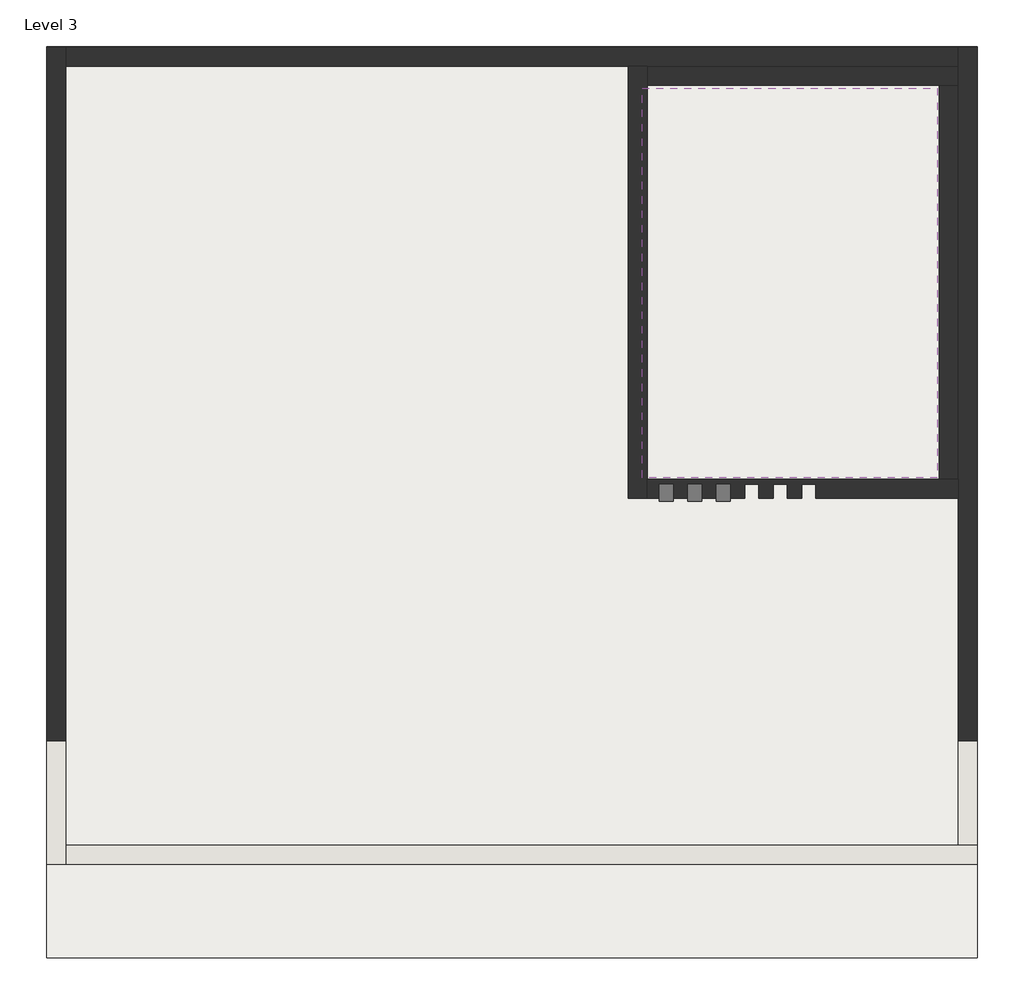
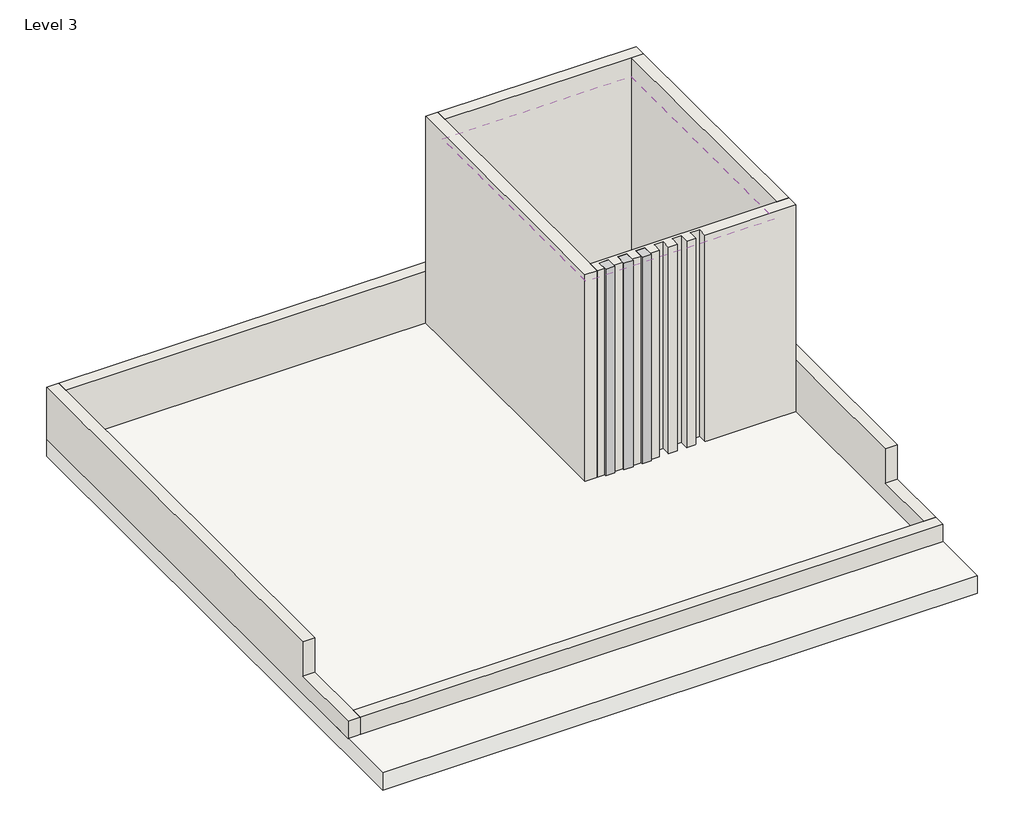
# One storey, incomplete: 8 walls, 3 proxies, 2 roofs.
"""IFC4 building model written with IfcOpenShell, lengths in millimetres."""

from ifc_helpers import new_model, si_unit, frame, origin, place, context, project, spatial, polyline, outline, extrude, faceted_brep, element, save

model = new_model("IFC4")

# Units and contexts
model_context = context("Model", 3, world=origin())
ifc_project = project(units=[si_unit("LENGTHUNIT", "METRE", prefix="MILLI")], contexts=[model_context])

# Site, building, storey
site = spatial("IfcSite", under=ifc_project)
building = spatial("IfcBuilding", under=site)
storey = spatial("IfcBuildingStorey", under=building, Name="Level 3", Elevation=7315.2)

# Proxies
placement = place(None, origin())
element("IfcBuildingElementProxy", 1, Name="Reveal", ObjectType="Reveal", at=placement, inside=storey, context=model_context, shape_type="SweptSolid", body=[
    extrude(outline(polyline([(-6259.9931367, 6437.3997066), (-6259.9931367, 6620.2797066), (-6107.5931367, 6620.2797066), (-6107.5931367, 6437.3997066), (-6259.9931367, 6437.3997066)])), frame((0.0, 0.0, 7620.0), z_axis=(0.0, 0.0, 1.0), x_axis=(1.0, 0.0, 0.0)), (0.0, 0.0, 1.0), 3657.6),
])
element("IfcBuildingElementProxy", 2, Name="Reveal", ObjectType="Reveal", at=placement, inside=storey, context=model_context, shape_type="SweptSolid", body=[
    extrude(outline(polyline([(-5955.1931367, 6437.3997066), (-5955.1931367, 6620.2797066), (-5802.7931367, 6620.2797066), (-5802.7931367, 6437.3997066), (-5955.1931367, 6437.3997066)])), frame((0.0, 0.0, 7620.0), z_axis=(0.0, 0.0, 1.0), x_axis=(1.0, 0.0, 0.0)), (0.0, 0.0, 1.0), 3657.6),
])
element("IfcBuildingElementProxy", 3, Name="Reveal", ObjectType="Reveal", at=placement, inside=storey, context=model_context, shape_type="SweptSolid", body=[
    extrude(outline(polyline([(-5650.3931367, 6437.3997066), (-5650.3931367, 6620.2797066), (-5497.9931367, 6620.2797066), (-5497.9931367, 6437.3997066), (-5650.3931367, 6437.3997066)])), frame((0.0, 0.0, 7620.0), z_axis=(0.0, 0.0, 1.0), x_axis=(1.0, 0.0, 0.0)), (0.0, 0.0, 1.0), 3657.6),
])

# Roofs
element("IfcRoof", 4, ObjectType="Generic - 12\"", at=placement, inside=storey, context=model_context, shape_type="SweptSolid", body=[
    extrude(outline(polyline([(-12813.1931367, 11300.8300502), (-2856.3931367, 11300.8300502), (-2856.3931367, 1552.6285778), (-12813.1931367, 1552.6285778), (-12813.1931367, 11300.8300502)])), frame((0.0, 0.0, 7315.2), z_axis=(0.0, 0.0, 1.0), x_axis=(1.0, 0.0, 0.0)), (0.0, 0.0, 1.0), 304.8),
])
element("IfcRoof", 5, ObjectType="Generic - 12\"", at=placement, inside=storey, context=model_context, shape_type="SweptSolid", body=[
    extrude(outline(polyline([(-6444.1431367, 10855.7297066), (-3288.1931367, 10855.7297066), (-3288.1931367, 6690.1297066), (-6444.1431367, 6690.1297066), (-6444.1431367, 10855.7297066)])), frame((0.0, 0.0, 10972.8), z_axis=(0.0, 0.0, 1.0), x_axis=(1.0, 0.0, 0.0)), (0.0, 0.0, 1.0), 304.8),
])

# Walls
element("IfcWall", 6, ObjectType="Generic - 8\"", at=placement, inside=storey, context=model_context, shape_type="Brep", body=[
    faceted_brep([(-12813.1931367, 11293.8797066, 7620.0), (-12813.1931367, 2556.2797066, 7620.0), (-12813.1931367, 2556.2797066, 7924.8), (-12813.1931367, 3877.0797066, 7924.8), (-12813.1931367, 3877.0797066, 8534.4), (-12813.1931367, 11293.8797066, 8534.4), (-12609.9931367, 11293.8797066, 7620.0), (-12609.9931367, 11293.8797066, 8534.4), (-12609.9931367, 11090.6797066, 8534.4), (-12609.9931367, 3877.0797066, 8534.4), (-12609.9931367, 3877.0797066, 7924.8), (-12609.9931367, 2759.4797066, 7924.8), (-12609.9931367, 2556.2797066, 7924.8), (-12609.9931367, 2556.2797066, 7620.0)], [[[0, 1, 2, 3, 4, 5]], [[6, 7, 8, 9, 10, 11, 12, 13]], [[2, 1, 13, 12]], [[0, 5, 7, 6]], [[1, 0, 6, 13]], [[5, 4, 9, 8, 7]], [[3, 2, 12, 11, 10]], [[4, 3, 10, 9]]]),
])
element("IfcWall", 7, ObjectType="Generic - 8\"", at=placement, inside=storey, context=model_context, shape_type="Brep", body=[
    faceted_brep([(-12609.9931367, 2556.2797066, 7315.2), (-2856.3931367, 2556.2797066, 7315.2), (-2856.3931367, 2556.2797066, 7924.8), (-12609.9931367, 2556.2797066, 7924.8), (-12609.9931367, 2556.2797066, 7620.0), (-12609.9931367, 2759.4797066, 7315.2), (-12609.9931367, 2759.4797066, 7924.8), (-3059.5931367, 2759.4797066, 7924.8), (-2856.3931367, 2759.4797066, 7924.8), (-2856.3931367, 2759.4797066, 7620.0), (-2856.3931367, 2759.4797066, 7315.2)], [[[0, 1, 2, 3, 4]], [[5, 6, 7, 8, 9, 10]], [[0, 4, 3, 6, 5]], [[2, 1, 10, 9, 8]], [[1, 0, 5, 10]], [[3, 2, 8, 7, 6]]]),
])
element("IfcWall", 8, ObjectType="Generic - 8\"", at=placement, inside=storey, context=model_context, shape_type="Brep", body=[
    faceted_brep([(-2856.3931367, 11293.8797066, 7620.0), (-2856.3931367, 11293.8797066, 8534.4), (-2856.3931367, 3877.0797066, 8534.4), (-2856.3931367, 3877.0797066, 7924.8), (-2856.3931367, 2759.4797066, 7924.8), (-2856.3931367, 2759.4797066, 7620.0), (-3059.5931367, 11293.8797066, 7620.0), (-3059.5931367, 2759.4797066, 7620.0), (-3059.5931367, 2759.4797066, 7924.8), (-3059.5931367, 3877.0797066, 7924.8), (-3059.5931367, 3877.0797066, 8534.4), (-3059.5931367, 11090.6797066, 8534.4), (-3059.5931367, 11293.8797066, 8534.4)], [[[0, 1, 2, 3, 4, 5]], [[6, 7, 8, 9, 10, 11, 12]], [[1, 0, 6, 12]], [[0, 5, 7, 6]], [[2, 1, 12, 11, 10]], [[3, 2, 10, 9]], [[4, 3, 9, 8]], [[5, 4, 8, 7]]]),
])
element("IfcWall", 9, ObjectType="Generic - 8\"", at=placement, inside=storey, context=model_context, shape_type="Brep", body=[
    faceted_brep([(-3059.5931367, 11293.8797066, 7315.2), (-12609.9931367, 11293.8797066, 7315.2), (-12609.9931367, 11293.8797066, 7620.0), (-12609.9931367, 11293.8797066, 8534.4), (-3059.5931367, 11293.8797066, 8534.4), (-3059.5931367, 11293.8797066, 7620.0), (-3059.5931367, 11090.6797066, 7315.2), (-3059.5931367, 11090.6797066, 8534.4), (-12609.9931367, 11090.6797066, 8534.4), (-12609.9931367, 11090.6797066, 7315.2)], [[[0, 1, 2, 3, 4, 5]], [[6, 7, 8, 9]], [[1, 0, 6, 9]], [[4, 3, 8, 7]], [[3, 2, 1, 9, 8]], [[0, 5, 4, 7, 6]]]),
])
element("IfcWall", 10, ObjectType="Generic - 8\"", at=placement, inside=storey, context=model_context, shape_type="Brep", body=[
    faceted_brep([(-6590.1931367, 11090.6797066, 11277.6), (-6590.1931367, 11090.6797066, 3962.4), (-6590.1931367, 6467.8797066, 3962.4), (-6590.1931367, 6467.8797066, 11277.6), (-6386.9931367, 11090.6797066, 3962.4), (-6386.9931367, 11090.6797066, 7315.2), (-6386.9931367, 11090.6797066, 11277.6), (-6386.9931367, 10887.4797066, 11277.6), (-6386.9931367, 6671.0797066, 11277.6), (-6386.9931367, 6467.8797066, 11277.6), (-6386.9931367, 6467.8797066, 3962.4), (-6386.9931367, 6671.0797066, 3962.4)], [[[0, 1, 2, 3]], [[4, 5, 6, 7, 8, 9, 10, 11]], [[2, 1, 4, 11, 10]], [[0, 3, 9, 8, 7, 6]], [[3, 2, 10, 9]], [[0, 6, 5, 4, 1]]]),
])
element("IfcWall", 11, ObjectType="Generic - 8\"", at=placement, inside=storey, context=model_context, shape_type="Brep", body=[
    faceted_brep([(-6386.9931367, 6467.8797066, 11277.6), (-6386.9931367, 6467.8797066, 3962.4), (-5345.5931367, 6467.8797066, 3962.4), (-5345.5931367, 6467.8797066, 11277.6), (-5497.9931367, 6467.8797066, 11277.6), (-5497.9931367, 6467.8797066, 7620.0), (-5650.3931367, 6467.8797066, 7620.0), (-5650.3931367, 6467.8797066, 11277.6), (-5802.7931367, 6467.8797066, 11277.6), (-5802.7931367, 6467.8797066, 7620.0), (-5955.1931367, 6467.8797066, 7620.0), (-5955.1931367, 6467.8797066, 11277.6), (-6107.5931367, 6467.8797066, 11277.6), (-6107.5931367, 6467.8797066, 7620.0), (-6259.9931367, 6467.8797066, 7620.0), (-6259.9931367, 6467.8797066, 11277.6), (-3059.5931367, 6467.8797066, 3962.4), (-3059.5931367, 6467.8797066, 11277.6), (-4583.5931367, 6467.8797066, 11277.6), (-4583.5931367, 6467.8797066, 3962.4), (-4431.1931367, 6467.8797066, 3962.4), (-4431.1931367, 6467.8797066, 7315.2), (-4278.7931367, 6467.8797066, 7315.2), (-4278.7931367, 6467.8797066, 3962.4), (-4126.3931367, 6467.8797066, 3962.4), (-4126.3931367, 6467.8797066, 7315.2), (-3973.9931367, 6467.8797066, 7315.2), (-3973.9931367, 6467.8797066, 3962.4), (-3821.5931367, 6467.8797066, 3962.4), (-3821.5931367, 6467.8797066, 7315.2), (-3669.1931367, 6467.8797066, 7315.2), (-3669.1931367, 6467.8797066, 3962.4), (-3542.1931367, 6467.8797066, 3962.4), (-3542.1931367, 6467.8797066, 7315.2), (-3389.7931367, 6467.8797066, 7315.2), (-3389.7931367, 6467.8797066, 3962.4), (-5193.1931367, 6467.8797066, 11277.6), (-5193.1931367, 6467.8797066, 3962.4), (-5040.7931367, 6467.8797066, 3962.4), (-5040.7931367, 6467.8797066, 11277.6), (-4888.3931367, 6467.8797066, 11277.6), (-4888.3931367, 6467.8797066, 3962.4), (-4735.9931367, 6467.8797066, 3962.4), (-4735.9931367, 6467.8797066, 11277.6), (-3059.5931367, 6671.0797066, 3962.4), (-6386.9931367, 6671.0797066, 3962.4), (-6386.9931367, 6671.0797066, 11277.6), (-3262.7931367, 6671.0797066, 11277.6), (-3059.5931367, 6671.0797066, 11277.6), (-3059.5931367, 6671.0797066, 7315.2), (-3389.7931367, 6620.2797066, 3962.4), (-3542.1931367, 6620.2797066, 3962.4), (-3669.1931367, 6620.2797066, 3962.4), (-3821.5931367, 6620.2797066, 3962.4), (-3973.9931367, 6620.2797066, 3962.4), (-4126.3931367, 6620.2797066, 3962.4), (-4278.7931367, 6620.2797066, 3962.4), (-4431.1931367, 6620.2797066, 3962.4), (-4583.5931367, 6620.2797066, 3962.4), (-4735.9931367, 6620.2797066, 3962.4), (-4888.3931367, 6620.2797066, 3962.4), (-5040.7931367, 6620.2797066, 3962.4), (-5193.1931367, 6620.2797066, 3962.4), (-5345.5931367, 6620.2797066, 3962.4), (-6259.9931367, 6620.2797066, 11277.6), (-6107.5931367, 6620.2797066, 11277.6), (-5955.1931367, 6620.2797066, 11277.6), (-5802.7931367, 6620.2797066, 11277.6), (-5650.3931367, 6620.2797066, 11277.6), (-5497.9931367, 6620.2797066, 11277.6), (-5345.5931367, 6620.2797066, 11277.6), (-5193.1931367, 6620.2797066, 11277.6), (-5040.7931367, 6620.2797066, 11277.6), (-4888.3931367, 6620.2797066, 11277.6), (-4735.9931367, 6620.2797066, 11277.6), (-4583.5931367, 6620.2797066, 11277.6), (-5802.7931367, 6620.2797066, 7620.0), (-5955.1931367, 6620.2797066, 7620.0), (-5497.9931367, 6620.2797066, 7620.0), (-5650.3931367, 6620.2797066, 7620.0), (-4431.1931367, 6620.2797066, 7315.2), (-4278.7931367, 6620.2797066, 7315.2), (-4126.3931367, 6620.2797066, 7315.2), (-3973.9931367, 6620.2797066, 7315.2), (-3821.5931367, 6620.2797066, 7315.2), (-3669.1931367, 6620.2797066, 7315.2), (-3542.1931367, 6620.2797066, 7315.2), (-3389.7931367, 6620.2797066, 7315.2), (-6107.5931367, 6620.2797066, 7620.0), (-6259.9931367, 6620.2797066, 7620.0)], [[[0, 1, 2, 3, 4, 5, 6, 7, 8, 9, 10, 11, 12, 13, 14, 15]], [[16, 17, 18, 19, 20, 21, 22, 23, 24, 25, 26, 27, 28, 29, 30, 31, 32, 33, 34, 35]], [[36, 37, 38, 39]], [[40, 41, 42, 43]], [[44, 45, 46, 47, 48, 49]], [[45, 44, 16, 35, 50, 51, 32, 31, 52, 53, 28, 27, 54, 55, 24, 23, 56, 57, 20, 19, 58, 59, 42, 41, 60, 61, 38, 37, 62, 63, 2, 1]], [[48, 47, 46, 0, 15, 64, 65, 12, 11, 66, 67, 8, 7, 68, 69, 4, 3, 70, 71, 36, 39, 72, 73, 40, 43, 74, 75, 18, 17]], [[1, 0, 46, 45]], [[16, 44, 49, 48, 17]], [[76, 77, 10, 9]], [[67, 76, 9, 8]], [[77, 76, 67, 66]], [[77, 66, 11, 10]], [[78, 79, 6, 5]], [[69, 78, 5, 4]], [[79, 78, 69, 68]], [[79, 68, 7, 6]], [[71, 62, 37, 36]], [[62, 71, 70, 63]], [[63, 70, 3, 2]], [[73, 60, 41, 40]], [[60, 73, 72, 61]], [[61, 72, 39, 38]], [[75, 58, 19, 18]], [[58, 75, 74, 59]], [[59, 74, 43, 42]], [[80, 81, 22, 21]], [[81, 56, 23, 22]], [[81, 80, 57, 56]], [[57, 80, 21, 20]], [[82, 83, 26, 25]], [[83, 54, 27, 26]], [[83, 82, 55, 54]], [[55, 82, 25, 24]], [[84, 85, 30, 29]], [[85, 52, 31, 30]], [[85, 84, 53, 52]], [[53, 84, 29, 28]], [[86, 87, 34, 33]], [[87, 50, 35, 34]], [[87, 86, 51, 50]], [[51, 86, 33, 32]], [[88, 89, 14, 13]], [[65, 88, 13, 12]], [[89, 88, 65, 64]], [[89, 64, 15, 14]]]),
])
element("IfcWall", 12, ObjectType="Generic - 8\"", at=placement, inside=storey, context=model_context, shape_type="Brep", body=[
    faceted_brep([(-6386.9931367, 10887.4797066, 7315.2), (-3262.7931367, 10887.4797066, 7315.2), (-3059.5931367, 10887.4797066, 7315.2), (-3059.5931367, 10887.4797066, 11277.6), (-3262.7931367, 10887.4797066, 11277.6), (-6386.9931367, 10887.4797066, 11277.6), (-6386.9931367, 11090.6797066, 7315.2), (-6386.9931367, 11090.6797066, 11277.6), (-3059.5931367, 11090.6797066, 11277.6), (-3059.5931367, 11090.6797066, 7315.2)], [[[0, 1, 2, 3, 4, 5]], [[6, 7, 8, 9]], [[2, 1, 0, 6, 9]], [[5, 4, 3, 8, 7]], [[3, 2, 9, 8]], [[0, 5, 7, 6]]]),
])
element("IfcWall", 13, ObjectType="Generic - 8\"", at=placement, inside=storey, context=model_context, shape_type="SweptSolid", body=[
    extrude(outline(polyline([(-3262.7931367, 6671.0797066), (-3262.7931367, 10887.4797066), (-3059.5931367, 10887.4797066), (-3059.5931367, 6671.0797066), (-3262.7931367, 6671.0797066)])), frame((0.0, 0.0, 7315.2), z_axis=(0.0, 0.0, 1.0), x_axis=(1.0, 0.0, 0.0)), (0.0, 0.0, 1.0), 3962.4),
])

save(model, "model.ifc")

# Revit data of these elements
# Type "Generic - 12\""
#   Assembly Code = "B1020"
#   Layers, outside or top first: 1' - 0" no material (function 1)
# Type "Generic - 8\""
#   Assembly Code = "B2010"
#   Layers, outside or top first: 0' - 8" no material (function 1)
# Element 4 (IfcRoof, "Generic - 12\"")
#   built-in parameter 1001705 = 25 (stored number, unit not read)
#   built-in parameter 1001710 = 33615
#   Phase Created = New Construction
#   Materials on its faces: "Default Roof"
# Element 5 (IfcRoof, "Generic - 12\"")
#   built-in parameter 1001705 = 37 (stored number, unit not read)
#   built-in parameter 1001701 = 12 (stored number, unit not read)
#   built-in parameter 1001710 = 33615
#   Phase Created = New Construction
#   Materials on its faces: "Default Roof"
# Elements 6, 8 (IfcWall, "Generic - 8\"")
#   built-in parameter 1001111 = 1' - 0"
#   Top Offset = 0' - 0"
#   Base Offset = 1' - 0"
#   Unconnected Height = 3' - 0"
#   wall height = 3' - 0"
#   Phase Created = New Construction
#   Base Constraint = Level 3
#   Materials on its faces: "Default Wall"
# Elements 7, 9 (IfcWall, "Generic - 8\"")
#   Top Offset = 0' - 0"
#   Base Offset = 0' - 0"
#   Unconnected Height = 4' - 0"
#   wall height = 4' - 0"
#   Phase Created = New Construction
#   Base Constraint = Level 3
#   Materials on its faces: "Default Wall"
# Elements 10, 11 (IfcWall, "Generic - 8\"")
#   built-in parameter 1001111 = -11' - 0"
#   Top Offset = 0' - 0"
#   Base Offset = -11' - 0"
#   Unconnected Height = 24' - 0"
#   wall height = 24' - 0"
#   Phase Created = New Construction
#   Base Constraint = Level 3
#   Materials on its faces: "Default Wall"
# Elements 12, 13 (IfcWall, "Generic - 8\"")
#   Top Offset = 0' - 0"
#   Base Offset = 0' - 0"
#   Unconnected Height = 13' - 0"
#   wall height = 13' - 0"
#   Phase Created = New Construction
#   Base Constraint = Level 3
#   Materials on its faces: "Default Wall"
# Materials
#   "Default Roof": colour RGB 88 101 114, transparency 0
#   "Default Wall": colour RGB 128 128 128, transparency 0
